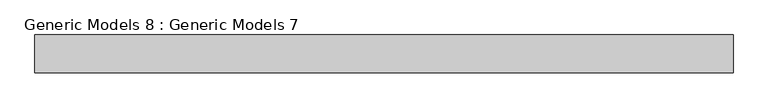
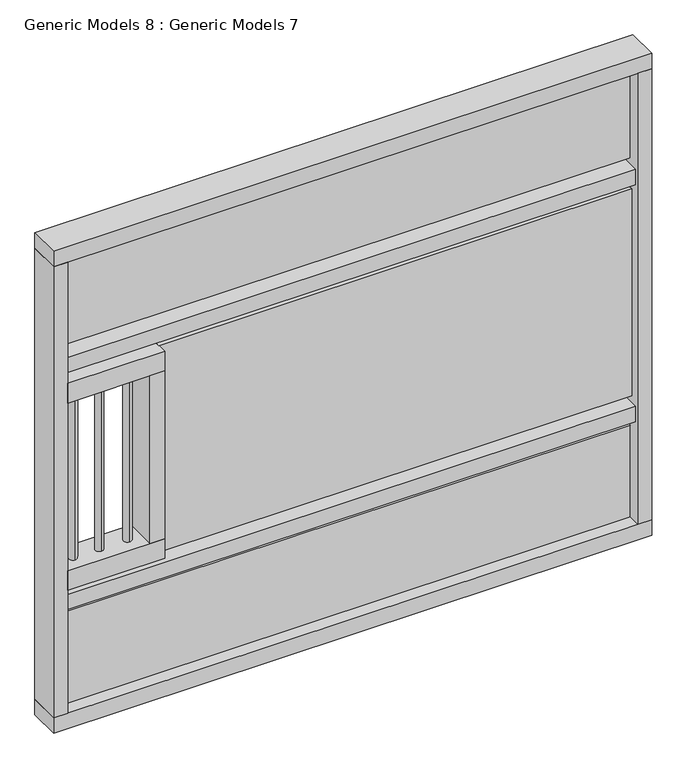
"""IFC4 building model written with IfcOpenShell, lengths in millimetres: proxy geometry, Generic Models 8 : Generic Models 7."""

from ifc_helpers import new_model, si_unit, point, frame, frame_2d, origin, place, context, project, spatial, polyline, circle_curve, trimmed, segment, composite_curve, outline, extrude, source, transform, mapped, element, save


def generic_models_8_generic_models_7_bb1c0133(model_context):
    return source(origin(), model_context, "Body", "SweptSolid", [
        extrude(outline(polyline([(-17595.8527072, -5389.7874709), (-17595.8527072, -5427.8893448), (-19082.8847028, -5427.8893448), (-19082.8847028, -5389.7874709), (-17595.8527072, -5389.7874709)])), frame((0.0, 0.0, 951.477172), z_axis=(0.0, 0.0, 1.0), x_axis=(1.0, 0.0, 0.0)), (0.0, 0.0, 1.0), 687.4014722),
        extrude(outline(composite_curve([segment(trimmed(circle_curve(frame_2d((-19343.8076942, -5413.1272599)), 12.7), [point((-19343.8076942, -5400.4272599))], [point((-19343.8076942, -5425.8272599))], False, "CARTESIAN"), True, "CONTINUOUS"), segment(trimmed(circle_curve(frame_2d((-19343.8076942, -5413.1272599)), 12.7), [point((-19343.8076942, -5425.8272599))], [point((-19343.8076942, -5400.4272599))], False, "CARTESIAN"), True, "CONTINUOUS")], self_intersect=False)), frame((0.0, 0.0, 1016.5786442), z_axis=(0.0, 0.0, 1.0), x_axis=(1.0, 0.0, 0.0)), (0.0, 0.0, 1.0), 564.5713558),
        extrude(outline(composite_curve([segment(trimmed(circle_curve(frame_2d((-19261.2576942, -5413.1272599)), 12.7), [point((-19261.2576942, -5400.4272599))], [point((-19261.2576942, -5425.8272599))], False, "CARTESIAN"), True, "CONTINUOUS"), segment(trimmed(circle_curve(frame_2d((-19261.2576942, -5413.1272599)), 12.7), [point((-19261.2576942, -5425.8272599))], [point((-19261.2576942, -5400.4272599))], False, "CARTESIAN"), True, "CONTINUOUS")], self_intersect=False)), frame((0.0, 0.0, 1016.5786442), z_axis=(0.0, 0.0, 1.0), x_axis=(1.0, 0.0, 0.0)), (0.0, 0.0, 1.0), 564.5713558),
        extrude(outline(composite_curve([segment(trimmed(circle_curve(frame_2d((-19172.3576942, -5413.1272599)), 12.7), [point((-19172.3576942, -5400.4272599))], [point((-19172.3576942, -5425.8272599))], False, "CARTESIAN"), True, "CONTINUOUS"), segment(trimmed(circle_curve(frame_2d((-19172.3576942, -5413.1272599)), 12.7), [point((-19172.3576942, -5425.8272599))], [point((-19172.3576942, -5400.4272599))], False, "CARTESIAN"), True, "CONTINUOUS")], self_intersect=False)), frame((0.0, 0.0, 1016.5786442), z_axis=(0.0, 0.0, 1.0), x_axis=(1.0, 0.0, 0.0)), (0.0, 0.0, 1.0), 564.5713558),
        extrude(outline(polyline([(-19082.8847028, -5358.3027976), (-19082.8847028, -5459.9027976), (-19128.8122097, -5459.9027976), (-19128.8122097, -5358.3027976), (-19082.8847028, -5358.3027976)])), frame((0.0, 0.0, 1016.5786442), z_axis=(0.0, 0.0, 1.0), x_axis=(1.0, 0.0, 0.0)), (0.0, 0.0, 1.0), 557.1985278),
        extrude(outline(polyline([(-19082.8847028, -5358.3027976), (-19082.8847028, -5459.9027976), (-19387.6847028, -5459.9027976), (-19387.6847028, -5358.3027976), (-19082.8847028, -5358.3027976)])), frame((0.0, 0.0, 1573.777172), z_axis=(0.0, 0.0, 1.0), x_axis=(1.0, 0.0, 0.0)), (0.0, 0.0, 1.0), 65.1014722),
        extrude(outline(polyline([(-19082.8847028, -5358.3027976), (-19082.8847028, -5459.9027976), (-19387.6847028, -5459.9027976), (-19387.6847028, -5358.3027976), (-19082.8847028, -5358.3027976)])), frame((0.0, 0.0, 951.477172), z_axis=(0.0, 0.0, 1.0), x_axis=(1.0, 0.0, 0.0)), (0.0, 0.0, 1.0), 65.1014722),
        extrude(outline(polyline([(-17595.8527072, -5371.189066), (-17595.8527072, -5447.389066), (-19387.6847028, -5447.389066), (-19387.6847028, -5371.189066), (-17595.8527072, -5371.189066)])), frame((0.0, 0.0, 1664.92529), z_axis=(0.0, 0.0, 1.0), x_axis=(1.0, 0.0, 0.0)), (0.0, 0.0, 1.0), 50.8),
        extrude(outline(polyline([(-17595.8527072, -5371.189066), (-17595.8527072, -5447.389066), (-19387.6847028, -5447.389066), (-19387.6847028, -5371.189066), (-17595.8527072, -5371.189066)])), frame((0.0, 0.0, 877.52529), z_axis=(0.0, 0.0, 1.0), x_axis=(1.0, 0.0, 0.0)), (0.0, 0.0, 1.0), 50.8),
        extrude(outline(polyline([(-17595.8527072, -5393.258566), (-17595.8527072, -5418.658566), (-19387.6847028, -5418.658566), (-19387.6847028, -5393.258566), (-17595.8527072, -5393.258566)])), frame((0.0, 0.0, 1737.2452447), z_axis=(0.0, 0.0, 1.0), x_axis=(1.0, 0.0, 0.0)), (0.0, 0.0, 1.0), 304.8),
        extrude(outline(polyline([(-17595.8527072, -5393.258566), (-17595.8527072, -5418.658566), (-19387.6847028, -5418.658566), (-19387.6847028, -5393.258566), (-17595.8527072, -5393.258566)])), frame((0.0, 0.0, 543.4452447), z_axis=(0.0, 0.0, 1.0), x_axis=(1.0, 0.0, 0.0)), (0.0, 0.0, 1.0), 304.8),
        extrude(outline(polyline([(-19431.568705, -5358.3027976), (-19387.6847028, -5358.3027976), (-19387.6847028, -5459.9027976), (-19431.568705, -5459.9027976), (-19431.568705, -5358.3027976)])), frame((0.0, 0.0, 543.4452447), z_axis=(0.0, 0.0, 1.0), x_axis=(1.0, 0.0, 0.0)), (0.0, 0.0, 1.0), 1498.6),
        extrude(outline(polyline([(-17595.8527072, -5358.3027976), (-17551.968705, -5358.3027976), (-17551.968705, -5459.9027976), (-17595.8527072, -5459.9027976), (-17595.8527072, -5358.3027976)])), frame((0.0, 0.0, 543.4452447), z_axis=(0.0, 0.0, 1.0), x_axis=(1.0, 0.0, 0.0)), (0.0, 0.0, 1.0), 1498.6),
        extrude(outline(polyline([(-17551.968705, -5358.3027976), (-17551.968705, -5459.9027976), (-19431.568705, -5459.9027976), (-19431.568705, -5358.3027976), (-17551.968705, -5358.3027976)])), frame((0.0, 0.0, 492.6452447), z_axis=(0.0, 0.0, 1.0), x_axis=(1.0, 0.0, 0.0)), (0.0, 0.0, 1.0), 50.8),
        extrude(outline(polyline([(-17551.968705, -5358.3027976), (-17551.968705, -5459.9027976), (-19431.568705, -5459.9027976), (-19431.568705, -5358.3027976), (-17551.968705, -5358.3027976)])), frame((0.0, 0.0, 2042.0452447), z_axis=(0.0, 0.0, 1.0), x_axis=(1.0, 0.0, 0.0)), (0.0, 0.0, 1.0), 50.8),
    ])


if __name__ == "__main__":
    model = new_model("IFC4")
    model_context = context("Model", 3, world=origin())
    ifc_project = project(units=[si_unit("LENGTHUNIT", "METRE", prefix="MILLI")], contexts=[model_context])
    site = spatial("IfcSite", under=ifc_project)
    building = spatial("IfcBuilding", under=site)
    placement = place(None, origin())
    generic_models_8_generic_models_7_shape = generic_models_8_generic_models_7_bb1c0133(model_context)
    element("IfcBuildingElementProxy", 1, Name="Generic Models 8 : Generic Models 7", ObjectType="Generic Models 8 : Generic Models 7", at=placement, inside=building, context=model_context, shape_type="MappedRepresentation", body=[
        mapped(generic_models_8_generic_models_7_shape, transform((0.0, 0.0, 0.0), x_axis=(1.0, 0.0, 0.0), y_axis=(0.0, 1.0, 0.0), z_axis=(0.0, 0.0, 1.0))),
    ])
    save(model, "model.ifc")

# Revit data of these elements
# Element 1 (IfcBuildingElementProxy, "Generic Models 8 : Generic Models 7")
#   Materials on its faces: "Damp-proofing", "Gypsum Wall Board", "Wood Planks"
# Materials
#   "Damp-proofing": class "Generic", colour RGB 17 17 17, transparency 0, Description = "Damp-proofing", Cost = 0
#   "Gypsum Wall Board": class "Generic", colour RGB 228 228 228, transparency 0, Description = "Gypsum Wall Board", Cost = 0
#   "Wood Planks": class "Wood", colour RGB 129 72 39, transparency 0, Description = "Physical material.", Cost = 0
